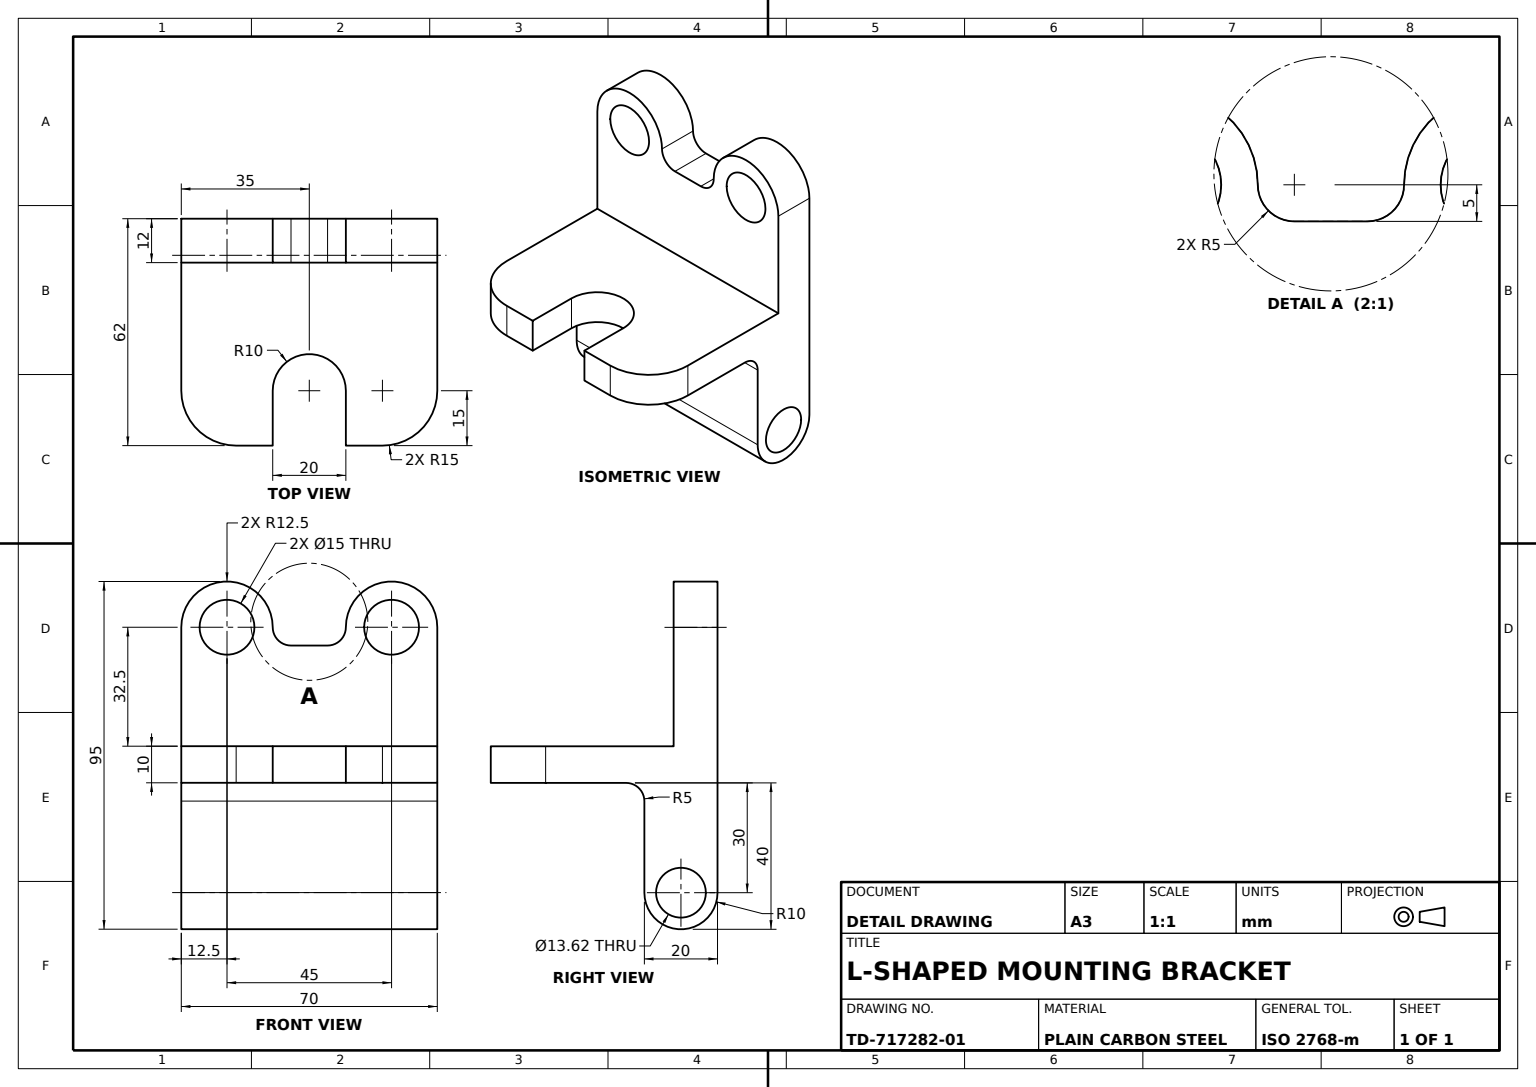
SolidWorks part; units mm, degrees
material "Plain Carbon Steel"
ref_plane "Front Plane" through (0, 0, 0) normal (0, 0, 1) x (1, 0, 0)
ref_plane "Top Plane" through (0, 0, 0) normal (0, 1, 0) x (1, 0, 0)
ref_plane "Right Plane" through (0, 0, 0) normal (1, 0, 0) x (0, 0, -1)
sketch "Base Plate Sketch" plane through (0, 0, 0) normal (0, 1, 0) x (1, 0, 0)
  line L0 (47, 75.6877) -> (47, -10.7753) construction
  line L1 (0, 0) -> (47, 0)
  line L2 (0, 0) -> (0, 70)
  line L3 (0, 70) -> (47, 70)
  line L4 (62, 15) -> (62, 25)
  line L5 (47, 45) -> (62, 45)
  line L6 (87.8232, 45) -> (87.8232, 25) construction
  line L7 (62, 25) -> (47, 25)
  line L8 (62, 45) -> (62, 55)
  arc A0 (47, 45) -> (47, 25) centre (47, 35) ccw
  arc A1 (47, 70) -> (62, 55) centre (47, 55) cw
  arc A2 (47, 0) -> (62, 15) centre (47, 15) ccw
  point P16 (62, 70)
  point P19 (62, 0)
  dimension "D7" = 20
  dimension "D4" = 15
  dimension "D1" = 62
  dimension "D2" = 70
  dimension "D3" = 15
  dimension "D5" = 25.8232
  dimension "D8" = 35
extrude "Base Plate" add sketch "Base Plate Sketch" along normal blind 10
sketch "Support Boss Sketch" plane through (0, 0, 0) normal (0, 0, 1) x (1, 0, 0)
  line L0 (0, 0) -> (0, -30)
  line L1 (20, -30) -> (20, -5)
  line L2 (47, 10) -> (47, 0) construction
  line L3 (0, 0) -> (25, 0)
  line L4 (0, 0) -> (47, 0) construction
  arc A0 (0, -30) -> (20, -30) centre (10, -30) ccw
  circle A1 centre (10, -30) radius 6.8107
  arc A2 (25, 0) -> (20, -5) centre (25, -5) ccw
  dimension "D2" = 10
  dimension "D1" = 5
  dimension "D3" = 13.6214
  dimension "D4" = 27
  dimension "D5" = 30
extrude "Support Boss" add sketch "Support Boss Sketch" against normal through all
sketch "Flange Sketch" plane through (0, 0, 0) normal (-1, 0, 0) x (0, 0, 1)
  line L0 (-70, 10) -> (-70, 42.5)
  line L1 (0, 10) -> (0, 42.5)
  line L2 (-92.8811, 42.5) -> (14.5927, 42.5) construction
  line L3 (-40, 37.5) -> (-30, 37.5)
  line L4 (-70, 10) -> (0, 10) construction
  line L5 (-70, 10) -> (0, 10)
  arc A0 (0, 42.5) -> (-25, 42.5) centre (-12.5, 42.5) ccw
  arc A1 (-25, 42.5) -> (-30, 37.5) centre (-30, 42.5) cw
  arc A2 (-45, 42.5) -> (-70, 42.5) centre (-57.5, 42.5) ccw
  arc A3 (-45, 42.5) -> (-40, 37.5) centre (-40, 42.5) ccw
  dimension "D1" = 12.5
  dimension "D3" = 12.5
  dimension "D6" = 5
  dimension "D2" = 32.5
  dimension "D4" = 32.5
extrude "Flange" add sketch "Flange Sketch" against normal blind 12
sketch "Flange Slot Sketch" plane through (12, 0, 0) normal (1, 0, 0) x (0, 0, -1)
  circle A0 centre (12.5, 42.5) radius 7.5
  circle A1 centre (57.5, 42.5) radius 7.5
  dimension "D1" = 15
extrude "Flange Slot Cut" cut sketch "Flange Slot Sketch" against normal blind 12
